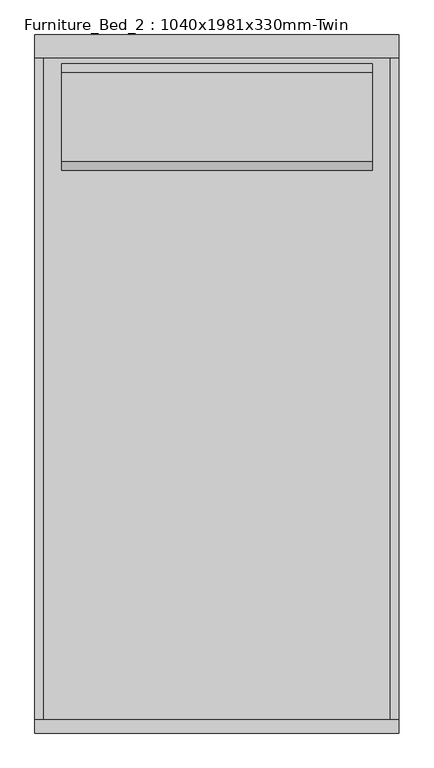
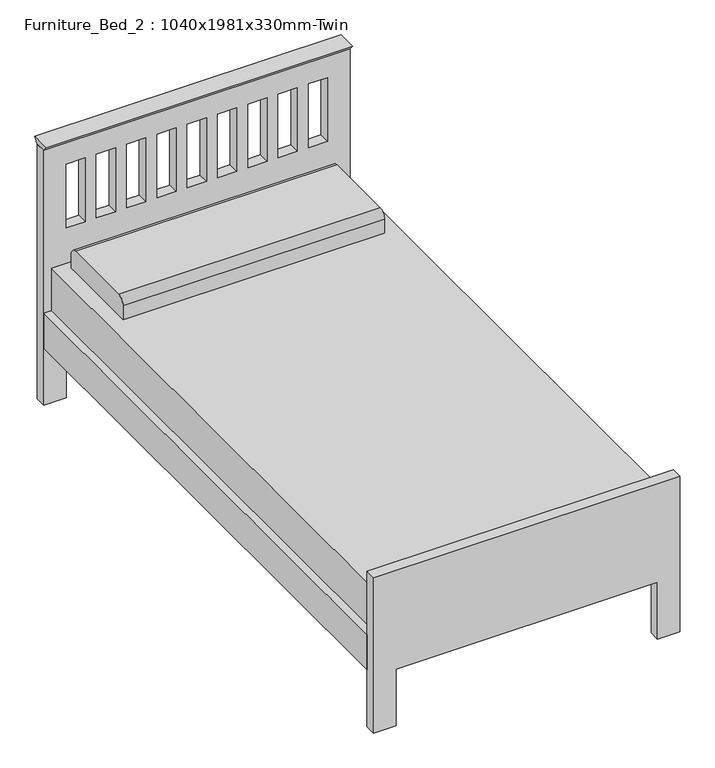
"""IFC4 building model written with IfcOpenShell, lengths in millimetres: furniture geometry, Furniture_Bed_2 : 1040x1981x330mm-Twin."""

from ifc_helpers import new_model, si_unit, point, frame, frame_2d, origin, place, context, project, spatial, polyline, circle_curve, trimmed, segment, composite_curve, outline, extrude, source, transform, mapped, element, save


def furniture_bed_2_1040x1981x330mm_twin_f17094d1(model_context):
    return source(origin(), model_context, "Body", "SweptSolid", [
        extrude(outline(polyline([(914.4, 501.9168067), (914.4, -539.5365546), (0.0, -539.5365546), (0.0, -463.55), (203.2, -463.55), (203.2, 425.45), (0.0, 425.45), (0.0, 501.9168067), (914.4, 501.9168067)]), holes=[polyline([(838.2, -398.6388889), (609.6, -398.6388889), (609.6, -463.55), (838.2, -463.55), (838.2, -398.6388889)]), polyline([(838.2, -295.6277778), (609.6, -295.6277778), (609.6, -360.5388889), (838.2, -360.5388889), (838.2, -295.6277778)]), polyline([(838.2, -192.6166667), (609.6, -192.6166667), (609.6, -257.5277778), (838.2, -257.5277778), (838.2, -192.6166667)]), polyline([(838.2, -89.6055556), (609.6, -89.6055556), (609.6, -154.5166667), (838.2, -154.5166667), (838.2, -89.6055556)]), polyline([(838.2, 116.4166667), (609.6, 116.4166667), (609.6, 51.5055556), (838.2, 51.5055556), (838.2, 116.4166667)]), polyline([(838.2, 219.4277778), (609.6, 219.4277778), (609.6, 154.5166667), (838.2, 154.5166667), (838.2, 219.4277778)]), polyline([(838.2, 322.4388889), (609.6, 322.4388889), (609.6, 257.5277778), (838.2, 257.5277778), (838.2, 322.4388889)]), polyline([(838.2, 425.45), (609.6, 425.45), (609.6, 360.5388889), (838.2, 360.5388889), (838.2, 425.45)]), polyline([(838.2, 13.4055556), (609.6, 13.4055556), (609.6, -51.5055556), (838.2, -51.5055556), (838.2, 13.4055556)])]), frame((0.0, -38.1, 0.0), z_axis=(0.0, 1.0, 0.0), x_axis=(0.0, 0.0, 1.0)), (0.0, 0.0, 1.0), 38.1),
        extrude(outline(polyline([(0.0, -463.55), (203.2, -463.55), (203.2, 425.45), (0.0, 425.45), (0.0, 501.65), (558.8, 501.65), (558.8, -539.75), (0.0, -539.75), (0.0, -463.55)])), frame((0.0, -1981.2, 0.0), z_axis=(0.0, 1.0, 0.0), x_axis=(0.0, 0.0, 1.0)), (0.0, 0.0, 1.0), 38.1),
        extrude(outline(polyline([(-539.75, -1943.1), (-539.75, -38.1), (-514.35, -38.1), (-514.35, -1943.1), (-539.75, -1943.1)])), frame((0.0, 0.0, 203.5755296), z_axis=(0.0, 0.0, 1.0), x_axis=(1.0, 0.0, 0.0)), (0.0, 0.0, 1.0), 127.0),
        extrude(outline(polyline([(476.25, -1943.1), (476.25, -38.1), (501.65, -38.1), (501.65, -1943.1), (476.25, -1943.1)])), frame((0.0, 0.0, 203.0994861), z_axis=(0.0, 0.0, 1.0), x_axis=(1.0, 0.0, 0.0)), (0.0, 0.0, 1.0), 127.0),
        extrude(outline(polyline([(476.25, -38.1), (476.25, -1943.1), (-514.35, -1943.1), (-514.35, -38.1), (476.25, -38.1)])), frame((0.0, 0.0, 228.6), z_axis=(0.0, 0.0, 1.0), x_axis=(1.0, 0.0, 0.0)), (0.0, 0.0, 1.0), 254.0),
        extrude(outline(composite_curve([segment(polyline([(-373.2486637, 482.6), (-373.2486637, 533.4)]), True, "CONTINUOUS"), segment(trimmed(circle_curve(frame_2d((-347.8486637, 533.4)), 25.4), [point((-373.2486637, 533.4))], [point((-347.8486637, 558.8))], False, "CARTESIAN"), True, "CONTINUOUS"), segment(polyline([(-347.8486637, 558.8), (-93.8486637, 558.8)]), True, "CONTINUOUS"), segment(trimmed(circle_curve(frame_2d((-93.8486637, 533.4)), 25.4), [point((-93.8486637, 558.8))], [point((-68.4486637, 533.4))], False, "CARTESIAN"), True, "CONTINUOUS"), segment(polyline([(-68.4486637, 533.4), (-68.4486637, 482.6), (-373.2486637, 482.6)]), True, "CONTINUOUS")], self_intersect=False)), frame((-463.55, 0.0, 0.0), z_axis=(1.0, 0.0, 0.0), x_axis=(0.0, 1.0, 0.0)), (0.0, 0.0, 1.0), 889.0),
        extrude(outline(polyline([(-38.1, 914.4), (-51.9545455, 933.45), (13.8545455, 933.45), (0.0, 914.4), (-38.1, 914.4)])), frame((-539.5365546, 0.0, 0.0), z_axis=(1.0, 0.0, 0.0), x_axis=(0.0, 1.0, 0.0)), (0.0, 0.0, 1.0), 1041.4533613),
    ])


if __name__ == "__main__":
    model = new_model("IFC4")
    model_context = context("Model", 3, world=origin())
    ifc_project = project(units=[si_unit("LENGTHUNIT", "METRE", prefix="MILLI")], contexts=[model_context])
    site = spatial("IfcSite", under=ifc_project)
    building = spatial("IfcBuilding", under=site)
    placement = place(None, origin())
    furniture_bed_2_1040x1981x330mm_twin_shape = furniture_bed_2_1040x1981x330mm_twin_f17094d1(model_context)
    element("IfcFurniture", 1, ObjectType="Furniture_Bed_2 : 1040x1981x330mm-Twin", at=placement, inside=building, context=model_context, shape_type="MappedRepresentation", body=[
        mapped(furniture_bed_2_1040x1981x330mm_twin_shape, transform((0.0, 0.0, 0.0), x_axis=(1.0, 0.0, 0.0), y_axis=(0.0, 1.0, 0.0), z_axis=(0.0, 0.0, 1.0))),
    ])
    save(model, "model.ifc")

# Revit data of these elements
# Type "Furniture_Bed_2 : 1040x1981x330mm-Twin"
#   Keynote = "N"
#   Length = 1981.2 mm
#   Width = 1041.4 mm
#   Material Frame = Wood - Birch
#   Material Mattress = Textile - White
#   Default Elevation = 0
# Element 1 (IfcFurniture, "Furniture_Bed_2 : 1040x1981x330mm-Twin")
#   Materials on its faces: "Wood - Birch", "Textile - White"
# Materials
#   "Wood - Birch": colour RGB 210 159 95, transparency 0
#   "Textile - White": class "Fabric", colour RGB 247 247 239, transparency 0
